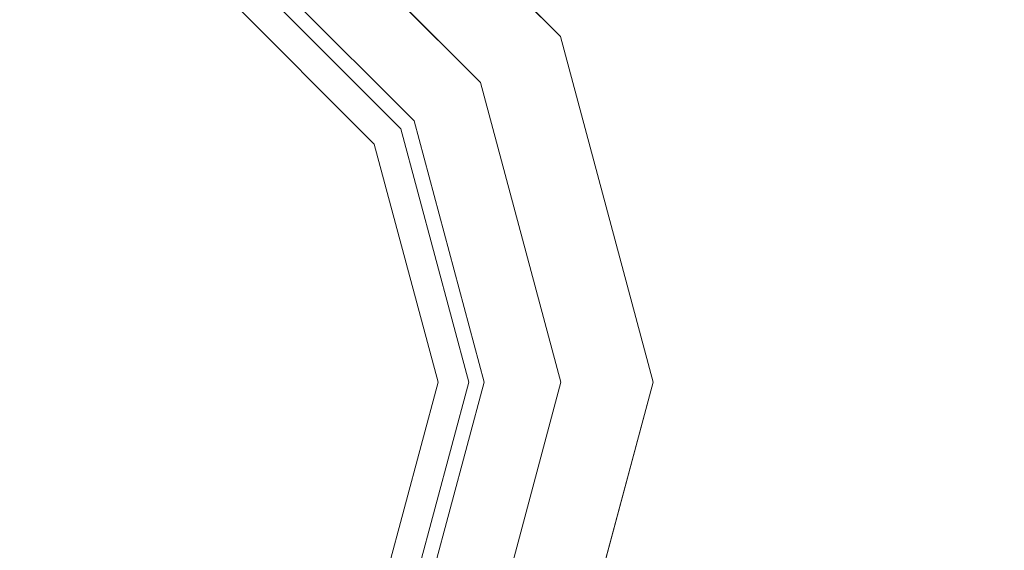
# Model space of a CAD drawing. Units: inches. Extents: x 375 to 1122, y 27 to 1069.
# Tile 102 of 155: x 713.015 to 720.91, y 867.921 to 872.174. Entities that reach past the tile are written whole.
import ezdxf

# ---------------------------------------------------------------- set-up
doc = ezdxf.new("R2010")
doc.units = ezdxf.units.IN
doc.layers.add('A-ANNO-DIMS', color=2, linetype='Continuous', lineweight=18)
doc.layers.add('Furniture', color=30, linetype='Continuous', lineweight=18)
doc.styles.get("Standard").update_dxf_attribs({"font": 'arial.ttf'})
doc.dimstyles.new('ISO-25', dxfattribs={"dimtxt": 12, "dimasz": 2.5, "dimexe": 1.5, "dimexo": 1.5, "dimtad": 1, "dimdec": 1, "dimlunit": 3, "dimtxsty": 'Standard', "dimblk": 'ARCHTICK', "dimcen": 2.5, "dimadec": 0, "dimazin": 0, "dimtfac": 1, "dimtdec": 1, "dimtmove": 0, "dimatfit": 3, "dimfxl": 1.5, "dimfxlon": 1, "dimarcsym": 0})

# ---------------------------------------------------------------- blocks, each defined once
blk = doc.blocks.new('A$C403C54AD')
at = {"linetype": 'ByBlock'}
for points, invisible_edges in [([(1.72651, 0.82864, -0.00874), (1.72651, 0.81017, -0.00874), (1.66648, 0.79408, -0.00874), (1.65725, 0.81008, -0.00874)], 5), ([(1.72651, 0.79478, -0.02259), (1.72651, 0.82864, -0.01335), (1.65725, 0.81008, -0.01335), (1.67418, 0.78075, -0.02259)], 5), ([(1.79578, 0.81008, -0.00874), (1.78654, 0.79408, -0.00874), (1.72651, 0.81017, -0.00874), (1.72651, 0.82864, -0.00874)], 5), ([(1.77884, 0.78075, -0.02259), (1.79578, 0.81008, -0.01335), (1.72651, 0.82864, -0.01335), (1.72651, 0.79478, -0.02259)], 5), ([(1.65725, 0.81008, -0.00874), (1.66648, 0.79408, -0.00874), (1.62254, 0.75014, -0.00874), (1.60654, 0.75938, -0.00874)], 5), ([(1.67418, 0.78075, -0.02259), (1.65725, 0.81008, -0.01335), (1.60654, 0.75938, -0.01335), (1.63587, 0.74244, -0.02259)], 5), ([(1.72651, 0.81017, -0.00874), (1.72651, 0.7917, -0.01489), (1.67572, 0.77809, -0.01489), (1.66648, 0.79408, -0.00874)], 5), ([(1.78654, 0.79408, -0.00874), (1.7773, 0.77809, -0.01489), (1.72651, 0.7917, -0.01489), (1.72651, 0.81017, -0.00874)], 5), ([(1.66648, 0.79408, -0.00874), (1.67572, 0.77809, -0.01489), (1.63853, 0.74091, -0.01489), (1.62254, 0.75014, -0.00874)], 5), ([(1.72651, 0.78554, -0.03183), (1.72651, 0.79478, -0.02259), (1.67418, 0.78075, -0.02259), (1.6788, 0.77276, -0.03183)], 5), ([(1.77423, 0.77276, -0.03183), (1.77884, 0.78075, -0.02259), (1.72651, 0.79478, -0.02259), (1.72651, 0.78554, -0.03183)], 5), ([(1.72651, 0.7917, -0.01489), (1.72651, 0.69011, -0.01489), (1.72651, 0.69011, -0.01489), (1.67572, 0.77809, -0.01489)], 5), ([(1.7773, 0.77809, -0.01489), (1.72651, 0.69011, -0.01489), (1.72651, 0.69011, -0.01489), (1.72651, 0.7917, -0.01489)], 5), ([(1.6788, 0.77276, -0.03183), (1.67418, 0.78075, -0.02259), (1.63587, 0.74244, -0.02259), (1.64387, 0.73783, -0.03183)], 1), ([(1.67572, 0.77809, -0.01489), (1.72651, 0.69011, -0.01489), (1.72651, 0.69011, -0.01489), (1.63853, 0.74091, -0.01489)], 5), ([(1.81449, 0.74091, -0.01489), (1.72651, 0.69011, -0.01489), (1.72651, 0.69011, -0.01489), (1.7773, 0.77809, -0.01489)], 5), ([(1.63853, 0.74091, -0.01489), (1.72651, 0.69011, -0.01489), (1.72651, 0.69011, -0.01489), (1.62492, 0.69011, -0.01489)], 5), ([(1.8281, 0.69011, -0.01489), (1.72651, 0.69011, -0.01489), (1.72651, 0.69011, -0.01489), (1.81449, 0.74091, -0.01489)], 5)]:
    blk.add_3dface(points, dxfattribs=dict(at, invisible_edges=invisible_edges))
for points in [[(1.72651, 0.82864, -0.01335), (1.72651, 0.82864, -0.00874), (1.65725, 0.81008, -0.00874), (1.65725, 0.81008, -0.01335)], [(1.79578, 0.81008, -0.01335), (1.79578, 0.81008, -0.00874), (1.72651, 0.82864, -0.00874), (1.72651, 0.82864, -0.01335)], [(1.65725, 0.81008, -0.01335), (1.65725, 0.81008, -0.00874), (1.60654, 0.75938, -0.00874), (1.60654, 0.75938, -0.01335)]]:
    blk.add_3dface(points, dxfattribs=at)
blk = doc.blocks.new('_ArchTick')
at = {"color": 0, "linetype": 'ByBlock', "const_width": 0.15}
blk.add_lwpolyline([(-0.5, -0.5), (0.5, 0.5)], dxfattribs=at)
blk = doc.blocks.new('*D85')
at = {"layer": 'A-ANNO-DIMS', "color": 0, "lineweight": -2, "transparency": 16777216}
for p, q in [((401.5073, 868.5277), (398.5073, 868.5277)), ((400.0073, 814.5277), (400.0073, 868.5277)), ((401.5073, 814.5277), (398.5073, 814.5277))]:
    blk.add_line(p, q, dxfattribs=at)
at = {"layer": 'Defpoints', "color": 0, "transparency": 16777216}
for p in [(400.0073, 868.5277), (845.0073, 868.5277), (845.0073, 814.5277)]:
    blk.add_point(p, dxfattribs=at)
at = {"layer": 'A-ANNO-DIMS', "color": 0, "lineweight": -2, "transparency": 16777216, "xscale": 2.5, "yscale": 2.5, "zscale": 2.5}
for p, rotation in [((400.0073, 868.5277), 90), ((400.0073, 814.5277), 270)]:
    blk.add_blockref('_ArchTick', p, dxfattribs=dict(at, rotation=rotation))
at = {"layer": 'A-ANNO-DIMS', "color": 0, "transparency": 16777216, "insert": (393.2555, 841.5277), "char_height": 12, "attachment_point": 5, "rotation": 90}
blk.add_mtext('4\'-6"', dxfattribs=at)

msp = doc.modelspace()

# ---------------------------------------------------------------- block references
at = {"layer": 'Furniture', "xscale": 39.9918517141215, "yscale": 39.9918517141215, "zscale": 39.9918517141215, "rotation": 270}
msp.add_blockref('A$C403C54AD', (684.9549, 938.3156, 0.024), dxfattribs=at)

# ---------------------------------------------------------------- dimensions: what is measured, and where the dimension line sits
at = {"layer": 'A-ANNO-DIMS'}
dim = msp.add_linear_dim(base=(400.0073, 868.5277), p1=(845.0073, 814.5277), p2=(845.0073, 868.5277), angle=90, dimstyle='ISO-25', override={"dimdec": 1, "dimlfac": 1, "dimrnd": 0, "dimzin": 1, "dimdsep": 46, "dimlunit": 4, "dimfrac": 2}, dxfattribs=at)
dim.commit()
dim.dimension.update_dxf_attribs({"geometry": '*D85', "text_midpoint": (393.2555, 841.5277)})

doc.saveas('drawing.dxf')
